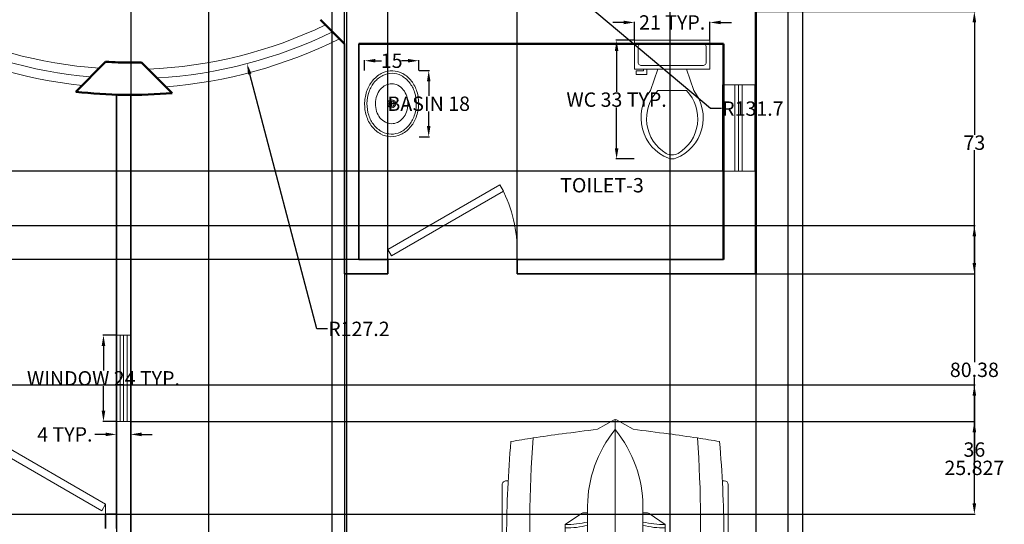
# Model space of a CAD drawing. Units: inches. Extents: x 1331 to 1798, y 701 to 1631.
# Tile 4 of 7: x 1524 to 1798, y 939 to 1079. Entities that reach past the tile are written whole.
import ezdxf

# ---------------------------------------------------------------- set-up
doc = ezdxf.new("R2010")
doc.units = ezdxf.units.IN
doc.header["$MEASUREMENT"] = 0
for name, color, linetype, lineweight in [('A-ANNO-DIMS', 2, 'Continuous', 18), ('A-AREA-IDEN', 7, 'Continuous', 18), ('A-EQPM-VEHI', 8, 'Continuous', 13), ('C-PROP', 7, 'Continuous', 25), ('DOORS', 241, 'Continuous', 18), ('INNER WALL', 50, 'Continuous', 35), ('OUTERWALL', 130, 'Continuous', 50), ('SANITARY', 1, 'Continuous', 18), ('VENTILATOR', 222, 'Continuous', 18), ('WINDOWS', 201, 'Continuous', 18)]:
    doc.layers.add(name, color=color, linetype=linetype, lineweight=lineweight)
doc.styles.get("Standard").update_dxf_attribs({"font": 'arial.ttf'})
doc.dimstyles.get("Standard").update_dxf_attribs({"dimtxt": 4, "dimasz": 3, "dimexe": 0.18, "dimexo": 0.0625, "dimgap": 0.09, "dimtad": 0, "dimtih": 1, "dimtoh": 1, "dimdec": 1, "dimzin": 0, "dimdsep": 46, "dimlunit": 3, "dimtxsty": 'Standard', "dimcen": 0.09, "dimadec": 0, "dimazin": 0, "dimtfac": 1, "dimtdec": 1, "dimtofl": 0, "dimtmove": 0, "dimatfit": 3, "dimfxl": 1, "dimtolj": 1, "dimtzin": 0, "dimarcsym": 0})

# ---------------------------------------------------------------- blocks, each defined once
blk = doc.blocks.new('*U12')
for p, q in [((0, 0), (0, -100)), ((750, 0), (750, -100))]:
    blk.add_line(p, q)
blk.add_lwpolyline([(0, 0), (649.5, 375), (671.4, 337.1), (21.9, -37.9)], close=True)
blk.add_arc((0, 0), 750, 0, 30)
blk = doc.blocks.new('*U14')
for p, q in [((0, 0), (0, 100)), ((750, 0), (750, 100))]:
    blk.add_line(p, q)
blk.add_lwpolyline([(0, 0), (649.5, -375), (671.4, -337.1), (21.9, 37.9)], close=True)
blk.add_arc((0, 0), 750, 330, 0)
blk = doc.blocks.new('Sink - Oval top')
for p, q in [((-1, 0), (1, 0)), ((0, 1), (0, -1))]:
    blk.add_line(p, q)
for points in [[(-12.23, 0.39, 0.117634), (-11.46, -3.36, 0.104469), (-8.88, -6.8, 0.090016), (-5.08, -9.07, 0.08192), (-0.32, -10.02, 0.08192), (4.49, -9.38, 0.090016), (8.42, -7.36, 0.104469), (11.22, -4.09, 0.117634), (12.23, -0.39, 0.117634), (11.46, 3.36, 0.104469), (8.88, 6.8, 0.090016), (5.08, 9.07, 0.08192), (0.32, 10.02, 0.08192), (-4.49, 9.38, 0.090016), (-8.42, 7.36, 0.104469), (-11.22, 4.09, 0.117634)], [(-11.29, 0.16, 0.118622), (-10.52, -3.25, 0.104678), (-8.07, -6.36, 0.089562), (-4.54, -8.37, 0.081185), (-0.13, -9.15, 0.081185), (4.3, -8.49, 0.089562), (7.89, -6.58, 0.104678), (10.42, -3.55, 0.118622), (11.29, -0.16, 0.118622), (10.52, 3.25, 0.104678), (8.07, 6.36, 0.089562), (4.54, 8.37, 0.081185), (0.13, 9.15, 0.081185), (-4.3, 8.49, 0.089562), (-7.89, 6.58, 0.104678), (-10.42, 3.55, 0.118622)], [(-7.42, 0.08, 0.118283), (-6.91, -2.17, 0.104607), (-5.29, -4.21, 0.089718), (-2.97, -5.53, 0.081436), (-0.07, -6.04, 0.081436), (2.84, -5.59, 0.089718), (5.2, -4.33, 0.104607), (6.86, -2.32, 0.118283), (7.42, -0.08, 0.118283), (6.91, 2.17, 0.104607), (5.29, 4.21, 0.089718), (2.97, 5.53, 0.081436), (0.07, 6.04, 0.081436), (-2.84, 5.59, 0.089718), (-5.2, 4.33, 0.104607), (-6.86, 2.32, 0.118283)]]:
    blk.add_lwpolyline(points, format="xyb", close=True)
for radius in [1.5, 1]:
    blk.add_circle((0, 0), radius)
blk = doc.blocks.new('*U17')
for p, q in [((21.1, 37.41), (21.1, 36.83)), ((46.55, 38.89), (22.35, 38.89)), ((47.8, 37.39), (47.8, 37.41)), ((135.45, 37.07), (135.45, 37.41)), ((136.7, 38.89), (160.9, 38.89)), ((162.15, 37.41), (162.15, 36.77)), ((87.99, 31.87), (74.76, 35.92)), ((134.31, 35.6), (119.29, 31.78)), ((70.03, 31.54), (86.41, 29.35)), ((186.47, -33.5), (186.47, 33.5)), ((188.4, -32.76), (188.4, 32.76)), ((138.42, 29.35), (157.25, 29.35)), ((186.47, 29.35), (167.01, 29.35)), ((164.52, 26.39), (164.52, -26.39)), ((32.27, 11.63), (36.13, 17.17)), ((36.13, 17.17), (50.94, 17.17)), ((32.12, 9.51), (32.12, 11.15)), ((58.92, -10.77), (58.92, 10.77)), ((66.55, -10.53), (66.55, 10.53)), ((186.47, -10.53), (186.47, 10.53)), ((29.77, 9.51), (51.68, 9.51)), ((82.74, 8.5), (82.74, -8.5)), ((3.27, 6.13), (0.1, 0.41)), ((0, 0), (51.68, 0)), ((0.1, -0.41), (3.27, -6.13)), ((29.77, -9.51), (51.68, -9.51)), ((32.12, -9.51), (32.12, -11.15)), ((32.27, -11.63), (36.13, -17.17)), ((36.13, -17.17), (50.94, -17.17)), ((86.41, -29.35), (70.03, -31.54)), ((157.25, -29.35), (138.42, -29.35)), ((167.01, -29.35), (186.47, -29.35)), ((87.99, -31.87), (74.76, -35.92)), ((134.31, -35.6), (119.29, -31.78)), ((21.1, -37.41), (21.1, -36.83)), ((135.45, -37.07), (135.45, -37.41)), ((162.15, -37.41), (162.15, -36.77)), ((46.55, -38.89), (22.35, -38.89)), ((47.8, -37.39), (47.8, -37.41)), ((136.7, -38.89), (160.9, -38.89))]:
    blk.add_line(p, q)
for centre, major_axis, ratio, start_param, end_param in [((41.19, -490.86), (0, 528.23), 0.842304, 0.00281, 0.075598), ((22.35, 37.41), (0, -1.48), 0.842304, 3.141593, 4.712389), ((64.48, -10555.62), (0, 10593.03), 0.842304, -0.013397, 0.002797), ((46.55, 37.41), (0, 1.48), 0.842304, -1.570796, 0), ((136.7, 37.41), (0, -1.48), 0.842304, 3.141593, 4.712389), ((160.9, 37.41), (0, 1.48), 0.842304, -1.570796, 0), ((180.63, 35.84), (0, 2.22), 0.842304, -0.013017, 1.249894), ((64.48, -10556.36), (0, 10595.31), 0.842304, -0.013397, -0.013017), ((183.98, 32.76), (0, -5.25), 0.842304, 1.570796, 3.128196), ((266.03, -27.52), (0, 313.31), 0.842304, 1.367076, 1.39176), ((64.48, -10555.62), (0, -10591.55), 0.842304, 3.133765, 3.140441), ((183.98, 33.5), (0, -2.96), 0.842304, 1.570796, 3.128196), ((135.29, 5.39), (0, 81.77), 0.842304, 1.245306, 1.50788), ((95.79, -3666.35), (0, -3698.24), 0.842304, 3.134049, 3.144098), ((259.18, -27.52), (0, -305.3), 0.842304, 4.528606, 4.561838), ((37.47, -593.96), (0, -623.33), 0.842304, 3.096046, 3.200911), ((134.4, 5.39), (0, -89.78), 0.842304, 4.449482, 4.652344), ((149.6, 2.8), (0, -79.58), 0.842304, 4.372215, 4.640744), ((17.08, 0), (0, 147.02), 0.842304, 4.511394, 4.913384), ((35.91, 0), (0, 147.02), 0.842304, 4.511394, 4.913384), ((167.01, 26.39), (0, 2.96), 0.842304, 0, 1.570796), ((-204.49, 52.4), (0, -250.96), 0.842304, 1.385369, 1.434372), ((13.04, 17.01), (0, 27.42), 0.842304, 4.435146, 4.718221), ((14.2, 17.01), (0, 27.42), 0.842304, 4.435146, 4.718221), ((50.79, 13.34), (6.34, -0.36), 0.603834, -1.395552, 1.581315), ((32.75, 11.15), (0, 0.74), 0.842304, 0.879714, 1.570796), ((29.77, -46.66), (0, 56.17), 0.842304, 0, 0.590319), ((0.62, 0), (0, -0.74), 0.842304, 4.131459, 5.293319), ((29.77, 46.66), (0, 56.17), 0.842304, 2.551274, 3.141593), ((-204.49, -52.4), (0, 250.96), 0.842304, -1.434372, -1.385369), ((13.04, -17.01), (0, -27.42), 0.842304, 1.564964, 1.848039), ((14.2, -17.01), (0, -27.42), 0.842304, 1.564964, 1.848039), ((149.6, -2.8), (0, -79.58), 0.842304, -1.499151, -1.230623), ((32.75, -11.15), (0, -0.74), 0.842304, 4.712389, 5.403472), ((134.4, -5.39), (0, -89.78), 0.842304, -1.510751, -1.307889), ((135.29, -5.39), (0, -81.77), 0.842304, -1.50788, -1.245306), ((259.18, 27.52), (0, 305.3), 0.842304, 1.721348, 1.754579), ((167.01, -26.39), (0, -2.96), 0.842304, 4.712389, 6.283185), ((266.03, 27.52), (0, 313.31), 0.842304, 1.749832, 1.774517), ((37.47, 593.96), (0, -623.33), 0.842304, -0.059319, 0.045547), ((95.79, 3666.35), (0, -3698.24), 0.842304, -0.002505, 0.007544), ((183.98, -33.5), (0, 2.96), 0.842304, 3.15499, 4.712389), ((183.98, -32.76), (0, -5.25), 0.842304, 0.013397, 1.570796), ((41.19, 490.86), (0, -528.23), 0.842304, -0.075598, -0.00281), ((64.48, 10555.62), (0, 10593.03), 0.842304, 3.138796, 3.15499), ((64.48, 10555.62), (0, -10591.55), 0.842304, 0.001152, 0.007828), ((180.63, -35.84), (0, -2.22), 0.842304, -1.249894, 0.013017), ((22.35, -37.41), (0, 1.48), 0.842304, 1.570796, 3.141593), ((46.55, -37.41), (0, -1.48), 0.842304, 0, 1.570796), ((136.7, -37.41), (0, -1.48), 0.842304, -1.570796, 0), ((160.9, -37.41), (0, 1.48), 0.842304, 3.141593, 4.712389), ((64.48, 10556.36), (0, 10595.31), 0.842304, 3.15461, 3.15499)]:
    blk.add_ellipse(centre, major_axis=major_axis, ratio=ratio, start_param=start_param, end_param=end_param)
at = {"extrusion": (0, 0, -1)}
blk.add_ellipse((50.79, -13.34), major_axis=(6.34, 0.36), ratio=0.603834, start_param=-1.395552, end_param=1.581315, dxfattribs=at)
blk = doc.blocks.new('Window - Wood Frame 36 in. Wide plan')
for p, q in [((0, 6), (0, 0)), ((0, 4.5), (36, 4.5)), ((36, 6), (36, 0)), ((0, 3), (36, 3)), ((0, 1.5), (36, 1.5))]:
    blk.add_line(p, q)
blk = doc.blocks.new('Toilet - top')
for p, q in [((9.5, -6), (9.5, -2)), ((-8, -8.5), (-8, -8)), ((-7, -8), (-7, -9.5)), ((-4, -8), (-6, -14)), ((4, -8), (6, -14)), ((-10, -8.5), (-8, -8.5)), ((-10, -9.5), (-10, -8.5)), ((-7, -9.5), (-10, -9.5)), ((4, -14), (-4, -14))]:
    blk.add_line(p, q)
blk.add_lwpolyline([(10.5, -8), (10.5, 0), (-10.5, 0), (-10.5, -8)], close=True)
for points in [[(-9.5, -2), (-9.5, -6)], [(8.5, -1), (-8.5, -1)], [(-8.5, -7), (8.5, -7)]]:
    blk.add_lwpolyline(points)
for centre, radius, start, end in [((-8.62, -1.88), 0.884, 81.8699, 188.1301), ((8.62, -1.88), 0.884, 351.8699, 98.1301), ((-8.62, -6.12), 0.884, 171.8699, 278.1301), ((8.62, -6.12), 0.884, 261.8699, 8.1301), ((3.52, -21.58), 12.17, 141.4691, 247.9714), ((4.2, -21.82), 11.33, 136.3677, 238.9468), ((-3.52, -21.58), 12.17, 292.0284, 38.5307), ((-4.2, -21.82), 11.33, 301.053, 43.6321), ((0, -27.88), 4, 245.7318, 294.2682), ((0, -29), 4, 254.8605, 285.1395)]:
    blk.add_arc(centre, radius, start, end)
blk = doc.blocks.new('VENT-FRAME-24IN')
for p, q in [((9, 24), (0, 24)), ((0, 24), (0, 0)), ((9, 0), (9, 24)), ((0, 0), (9, 0))]:
    blk.add_line(p, q)
blk = doc.blocks.new('*D26')
at = {"layer": 'A-ANNO-DIMS', "color": 0, "lineweight": -2, "transparency": 16777216}
for p, q in [((1550.6, 991.61), (1546.88, 991.61)), ((1547.06, 988.61), (1547.06, 981.77)), ((1547.06, 970.61), (1547.06, 977.46)), ((1550.6, 967.61), (1546.88, 967.61))]:
    blk.add_line(p, q, dxfattribs=at)
at = {"layer": 'A-ANNO-DIMS', "color": 0, "transparency": 16777216}
for points in [[(1546.56, 988.61), (1547.56, 988.61), (1547.06, 991.61)], [(1546.56, 970.61), (1547.56, 970.61), (1547.06, 967.61)]]:
    blk.add_solid(points, dxfattribs=at)
at = {"layer": 'Defpoints', "color": 0, "transparency": 16777216}
for p in [(1547.06, 991.61), (1550.66, 991.61), (1550.66, 967.61)]:
    blk.add_point(p, dxfattribs=at)
at = {"layer": 'A-ANNO-DIMS', "color": 0, "transparency": 16777216, "insert": (1547.06, 979.61), "char_height": 4, "attachment_point": 5}
blk.add_mtext('\\A1;WINDOW 24 TYP.', dxfattribs=at)
blk = doc.blocks.new('*D27')
at = {"layer": 'A-ANNO-DIMS', "color": 0, "lineweight": -2, "transparency": 16777216}
for p, q in [((1550.66, 967.55), (1550.66, 963.83)), ((1554.66, 967.55), (1554.66, 963.83)), ((1547.66, 964.01), (1544.66, 964.01)), ((1557.66, 964.01), (1560.66, 964.01))]:
    blk.add_line(p, q, dxfattribs=at)
at = {"layer": 'A-ANNO-DIMS', "color": 0, "transparency": 16777216}
for points in [[(1547.66, 964.51), (1547.66, 963.51), (1550.66, 964.01)], [(1557.66, 964.51), (1557.66, 963.51), (1554.66, 964.01)]]:
    blk.add_solid(points, dxfattribs=at)
at = {"layer": 'Defpoints', "color": 0, "transparency": 16777216}
for p in [(1550.66, 967.61), (1554.66, 967.61), (1550.66, 964.01)]:
    blk.add_point(p, dxfattribs=at)
at = {"layer": 'A-ANNO-DIMS', "color": 0, "transparency": 16777216, "insert": (1536.31, 964.01), "char_height": 4, "attachment_point": 5}
blk.add_mtext('\\A1;4 TYP.', dxfattribs=at)
blk = doc.blocks.new('*D36')
at = {"layer": 'A-ANNO-DIMS', "color": 0, "lineweight": -2, "transparency": 16777216}
for p, q in [((1634.88, 1065.25), (1637.76, 1065.25)), ((1637.58, 1062.25), (1637.58, 1058.2)), ((1637.58, 1049.83), (1637.58, 1053.88)), ((1634.88, 1046.83), (1637.76, 1046.83))]:
    blk.add_line(p, q, dxfattribs=at)
at = {"layer": 'A-ANNO-DIMS', "color": 0, "transparency": 16777216}
for points in [[(1637.08, 1062.25), (1638.08, 1062.25), (1637.58, 1065.25)], [(1637.08, 1049.83), (1638.08, 1049.83), (1637.58, 1046.83)]]:
    blk.add_solid(points, dxfattribs=at)
at = {"layer": 'Defpoints', "color": 0, "transparency": 16777216}
for p in [(1634.82, 1065.25), (1637.58, 1065.25), (1634.82, 1046.83)]:
    blk.add_point(p, dxfattribs=at)
at = {"layer": 'A-ANNO-DIMS', "color": 0, "transparency": 16777216, "insert": (1637.58, 1056.04), "char_height": 4, "attachment_point": 5}
blk.add_mtext('\\A1;BASIN 18', dxfattribs=at)
blk = doc.blocks.new('*D37')
at = {"layer": 'A-ANNO-DIMS', "color": 0, "lineweight": -2, "transparency": 16777216}
for p, q in [((1619.72, 1065.31), (1619.72, 1068.19)), ((1622.72, 1068.01), (1624.48, 1068.01)), ((1631.82, 1068.01), (1630.05, 1068.01)), ((1634.82, 1065.31), (1634.82, 1068.19))]:
    blk.add_line(p, q, dxfattribs=at)
at = {"layer": 'A-ANNO-DIMS', "color": 0, "transparency": 16777216}
for points in [[(1622.72, 1068.51), (1622.72, 1067.51), (1619.72, 1068.01)], [(1631.82, 1068.51), (1631.82, 1067.51), (1634.82, 1068.01)]]:
    blk.add_solid(points, dxfattribs=at)
at = {"layer": 'Defpoints', "color": 0, "transparency": 16777216}
for p in [(1619.72, 1068.01), (1619.72, 1065.25), (1634.82, 1065.25)]:
    blk.add_point(p, dxfattribs=at)
at = {"layer": 'A-ANNO-DIMS', "color": 0, "transparency": 16777216, "insert": (1627.27, 1068.01), "char_height": 4, "attachment_point": 5}
blk.add_mtext('\\A1;15', dxfattribs=at)
blk = doc.blocks.new('*D38')
at = {"layer": 'A-ANNO-DIMS', "color": 0, "lineweight": -2, "transparency": 16777216}
for p, q in [((1694.76, 1073.7), (1689.69, 1073.7)), ((1689.87, 1070.7), (1689.87, 1059.34)), ((1689.87, 1043.66), (1689.87, 1055.02)), ((1694.76, 1040.66), (1689.69, 1040.66))]:
    blk.add_line(p, q, dxfattribs=at)
at = {"layer": 'A-ANNO-DIMS', "color": 0, "transparency": 16777216}
for points in [[(1689.37, 1070.7), (1690.37, 1070.7), (1689.87, 1073.7)], [(1689.37, 1043.66), (1690.37, 1043.66), (1689.87, 1040.66)]]:
    blk.add_solid(points, dxfattribs=at)
at = {"layer": 'Defpoints', "color": 0, "transparency": 16777216}
for p in [(1689.87, 1073.7), (1694.83, 1073.7), (1694.83, 1040.66)]:
    blk.add_point(p, dxfattribs=at)
at = {"layer": 'A-ANNO-DIMS', "color": 0, "transparency": 16777216, "insert": (1689.87, 1057.18), "char_height": 4, "attachment_point": 5}
blk.add_mtext('\\A1;WC 33 TYP.', dxfattribs=at)
blk = doc.blocks.new('*D39')
at = {"layer": 'A-ANNO-DIMS', "color": 0, "lineweight": -2, "transparency": 16777216}
for p, q in [((1691.83, 1078.66), (1688.83, 1078.66)), ((1694.83, 1073.77), (1694.83, 1078.84)), ((1715.83, 1073.77), (1715.83, 1078.84)), ((1718.83, 1078.66), (1721.83, 1078.66))]:
    blk.add_line(p, q, dxfattribs=at)
at = {"layer": 'A-ANNO-DIMS', "color": 0, "transparency": 16777216}
for points in [[(1691.83, 1079.16), (1691.83, 1078.16), (1694.83, 1078.66)], [(1718.83, 1079.16), (1718.83, 1078.16), (1715.83, 1078.66)]]:
    blk.add_solid(points, dxfattribs=at)
at = {"layer": 'Defpoints', "color": 0, "transparency": 16777216}
for p in [(1715.83, 1078.66), (1694.83, 1073.7), (1715.83, 1073.7)]:
    blk.add_point(p, dxfattribs=at)
at = {"layer": 'A-ANNO-DIMS', "color": 0, "transparency": 16777216, "insert": (1705.33, 1078.66), "char_height": 4, "attachment_point": 5}
blk.add_mtext('\\A1;21 TYP.', dxfattribs=at)
blk = doc.blocks.new('*D55')
at = {"layer": 'A-ANNO-DIMS', "color": 0, "lineweight": -2, "transparency": 16777216}
for p, q in [((1554.66, 1190.15), (1554.66, 703.35)), ((1728.66, 1008.64), (1728.66, 703.35)), ((1557.66, 703.53), (1637.35, 703.53)), ((1725.66, 703.53), (1645.98, 703.53))]:
    blk.add_line(p, q, dxfattribs=at)
at = {"layer": 'A-ANNO-DIMS', "color": 0, "transparency": 16777216}
for points in [[(1557.66, 704.03), (1557.66, 703.03), (1554.66, 703.53)], [(1725.66, 704.03), (1725.66, 703.03), (1728.66, 703.53)]]:
    blk.add_solid(points, dxfattribs=at)
at = {"layer": 'Defpoints', "color": 0, "transparency": 16777216}
for p in [(1554.66, 1190.21), (1728.66, 1008.7), (1728.66, 703.53)]:
    blk.add_point(p, dxfattribs=at)
at = {"layer": 'A-ANNO-DIMS', "color": 0, "transparency": 16777216, "insert": (1641.66, 703.53), "char_height": 4, "attachment_point": 5}
blk.add_mtext('\\A1;174', dxfattribs=at)
blk = doc.blocks.new('*D61')
at = {"layer": 'A-ANNO-DIMS', "color": 0, "lineweight": -2, "transparency": 16777216}
for p, q in [((1554.663699, 1524.863082), (1554.663699, 703.345582)), ((1576.268161, 1524.863082), (1576.268161, 703.345582)), ((1551.663699, 703.525582), (1548.663699, 703.525582)), ((1579.268161, 703.525582), (1582.268161, 703.525582))]:
    blk.add_line(p, q, dxfattribs=at)
at = {"layer": 'A-ANNO-DIMS', "color": 0, "transparency": 16777216}
for points in [[(1551.663699, 704.025582), (1551.663699, 703.025582), (1554.663699, 703.525582)], [(1579.268161, 704.025582), (1579.268161, 703.025582), (1576.268161, 703.525582)]]:
    blk.add_solid(points, dxfattribs=at)
at = {"layer": 'Defpoints', "color": 0, "transparency": 16777216}
for p in [(1554.663699, 1524.925582), (1576.268161, 1524.925582), (1576.268161, 703.525582)]:
    blk.add_point(p, dxfattribs=at)
at = {"layer": 'A-ANNO-DIMS', "color": 0, "transparency": 16777216, "insert": (1565.46593, 703.525582), "char_height": 4, "attachment_point": 5}
blk.add_mtext('\\A1;21.604', dxfattribs=at)
blk = doc.blocks.new('*D69')
at = {"layer": 'A-ANNO-DIMS', "color": 0, "lineweight": -2, "transparency": 16777216}
for p, q in [((1614.66, 1376.86), (1614.66, 703.35)), ((1704.66, 1376.86), (1704.66, 703.35)), ((1617.66, 703.53), (1656.72, 703.53)), ((1701.66, 703.53), (1662.61, 703.53))]:
    blk.add_line(p, q, dxfattribs=at)
at = {"layer": 'A-ANNO-DIMS', "color": 0, "transparency": 16777216}
for points in [[(1617.66, 704.03), (1617.66, 703.03), (1614.66, 703.53)], [(1701.66, 704.03), (1701.66, 703.03), (1704.66, 703.53)]]:
    blk.add_solid(points, dxfattribs=at)
at = {"layer": 'Defpoints', "color": 0, "transparency": 16777216}
for p in [(1614.66, 1376.93), (1704.66, 1376.93), (1704.66, 703.53)]:
    blk.add_point(p, dxfattribs=at)
at = {"layer": 'A-ANNO-DIMS', "color": 0, "transparency": 16777216, "insert": (1659.66, 703.53), "char_height": 4, "attachment_point": 5}
blk.add_mtext('\\A1;90', dxfattribs=at)
blk = doc.blocks.new('*D71')
at = {"layer": 'A-ANNO-DIMS', "color": 0, "lineweight": -2, "transparency": 16777216}
for p, q in [((1506.66, 1376.86), (1506.66, 703.35)), ((1610.66, 1376.86), (1610.66, 703.35)), ((1509.66, 703.53), (1554.35, 703.53)), ((1607.66, 703.53), (1562.98, 703.53))]:
    blk.add_line(p, q, dxfattribs=at)
at = {"layer": 'A-ANNO-DIMS', "color": 0, "transparency": 16777216}
for points in [[(1509.66, 704.03), (1509.66, 703.03), (1506.66, 703.53)], [(1607.66, 704.03), (1607.66, 703.03), (1610.66, 703.53)]]:
    blk.add_solid(points, dxfattribs=at)
at = {"layer": 'Defpoints', "color": 0, "transparency": 16777216}
for p in [(1506.66, 1376.93), (1610.66, 1376.93), (1610.66, 703.53)]:
    blk.add_point(p, dxfattribs=at)
at = {"layer": 'A-ANNO-DIMS', "color": 0, "transparency": 16777216, "insert": (1558.66, 703.53), "char_height": 4, "attachment_point": 5}
blk.add_mtext('\\A1;104', dxfattribs=at)
blk = doc.blocks.new('*D75')
at = {"layer": 'A-ANNO-DIMS', "color": 0, "lineweight": -2, "transparency": 16777216}
for p, q in [((1418.66, 941.73), (1418.66, 703.35)), ((1550.66, 941.73), (1550.66, 703.35)), ((1421.66, 703.53), (1480.36, 703.53)), ((1547.66, 703.53), (1488.96, 703.53))]:
    blk.add_line(p, q, dxfattribs=at)
at = {"layer": 'A-ANNO-DIMS', "color": 0, "transparency": 16777216}
for points in [[(1421.66, 704.03), (1421.66, 703.03), (1418.66, 703.53)], [(1547.66, 704.03), (1547.66, 703.03), (1550.66, 703.53)]]:
    blk.add_solid(points, dxfattribs=at)
at = {"layer": 'Defpoints', "color": 0, "transparency": 16777216}
for p in [(1418.66, 941.79), (1550.66, 941.79), (1550.66, 703.53)]:
    blk.add_point(p, dxfattribs=at)
at = {"layer": 'A-ANNO-DIMS', "color": 0, "transparency": 16777216, "insert": (1484.66, 703.53), "char_height": 4, "attachment_point": 5}
blk.add_mtext('\\A1;132', dxfattribs=at)
blk = doc.blocks.new('*D79')
at = {"layer": 'A-ANNO-DIMS', "color": 0, "lineweight": -2, "transparency": 16777216}
for p, q in [((1554.73, 967.61), (1789.62, 967.61)), ((1789.44, 964.61), (1789.44, 956.83)), ((1789.44, 944.79), (1789.44, 952.57)), ((1550.73, 941.79), (1789.62, 941.79))]:
    blk.add_line(p, q, dxfattribs=at)
at = {"layer": 'A-ANNO-DIMS', "color": 0, "transparency": 16777216}
for points in [[(1788.94, 964.61), (1789.94, 964.61), (1789.44, 967.61)], [(1788.94, 944.79), (1789.94, 944.79), (1789.44, 941.79)]]:
    blk.add_solid(points, dxfattribs=at)
at = {"layer": 'Defpoints', "color": 0, "transparency": 16777216}
for p in [(1554.66, 967.61), (1789.44, 967.61), (1550.66, 941.79)]:
    blk.add_point(p, dxfattribs=at)
at = {"layer": 'A-ANNO-DIMS', "color": 0, "transparency": 16777216, "insert": (1789.44, 954.7), "char_height": 4, "attachment_point": 5}
blk.add_mtext('\\A1;25.827', dxfattribs=at)
blk = doc.blocks.new('*D82')
at = {"layer": 'A-ANNO-DIMS', "color": 0, "lineweight": -2, "transparency": 16777216}
for p, q in [((1418.73, 1022.17), (1789.62, 1022.17)), ((1789.44, 1019.17), (1789.44, 984.11)), ((1789.44, 944.79), (1789.44, 979.84)), ((1418.73, 941.79), (1789.62, 941.79))]:
    blk.add_line(p, q, dxfattribs=at)
at = {"layer": 'A-ANNO-DIMS', "color": 0, "transparency": 16777216}
for points in [[(1788.94, 1019.17), (1789.94, 1019.17), (1789.44, 1022.17)], [(1788.94, 944.79), (1789.94, 944.79), (1789.44, 941.79)]]:
    blk.add_solid(points, dxfattribs=at)
at = {"layer": 'Defpoints', "color": 0, "transparency": 16777216}
for p in [(1418.66, 1022.17), (1789.44, 1022.17), (1418.66, 941.79)]:
    blk.add_point(p, dxfattribs=at)
at = {"layer": 'A-ANNO-DIMS', "color": 0, "transparency": 16777216, "insert": (1789.44, 981.98), "char_height": 4, "attachment_point": 5}
blk.add_mtext('\\A1;80.38', dxfattribs=at)
blk = doc.blocks.new('*D84')
at = {"layer": 'A-ANNO-DIMS', "color": 0, "lineweight": -2, "transparency": 16777216}
for p, q in [((1493.13, 977.79), (1789.62, 977.79)), ((1789.44, 974.79), (1789.44, 961.92)), ((1789.44, 944.79), (1789.44, 957.65)), ((1493.13, 941.79), (1789.62, 941.79))]:
    blk.add_line(p, q, dxfattribs=at)
at = {"layer": 'A-ANNO-DIMS', "color": 0, "transparency": 16777216}
for points in [[(1788.94, 974.79), (1789.94, 974.79), (1789.44, 977.79)], [(1788.94, 944.79), (1789.94, 944.79), (1789.44, 941.79)]]:
    blk.add_solid(points, dxfattribs=at)
at = {"layer": 'Defpoints', "color": 0, "transparency": 16777216}
for p in [(1493.07, 977.79), (1789.44, 977.79), (1493.07, 941.79)]:
    blk.add_point(p, dxfattribs=at)
at = {"layer": 'A-ANNO-DIMS', "color": 0, "transparency": 16777216, "insert": (1789.44, 959.79), "char_height": 4, "attachment_point": 5}
blk.add_mtext('\\A1;36', dxfattribs=at)
blk = doc.blocks.new('*D85')
at = {"layer": 'A-ANNO-DIMS', "color": 0, "lineweight": -2, "transparency": 16777216}
for p, q in [((1614.16, 1008.64), (1614.16, 703.35)), ((1728.66, 1008.64), (1728.66, 703.35)), ((1617.16, 703.53), (1664.75, 703.53)), ((1725.66, 703.53), (1678.08, 703.53))]:
    blk.add_line(p, q, dxfattribs=at)
at = {"layer": 'A-ANNO-DIMS', "color": 0, "transparency": 16777216}
for points in [[(1617.16, 704.03), (1617.16, 703.03), (1614.16, 703.53)], [(1725.66, 704.03), (1725.66, 703.03), (1728.66, 703.53)]]:
    blk.add_solid(points, dxfattribs=at)
at = {"layer": 'Defpoints', "color": 0, "transparency": 16777216}
for p in [(1614.16, 1008.7), (1728.66, 1008.7), (1728.66, 703.53)]:
    blk.add_point(p, dxfattribs=at)
at = {"layer": 'A-ANNO-DIMS', "color": 0, "transparency": 16777216, "insert": (1671.41, 703.53), "char_height": 4, "attachment_point": 5}
blk.add_mtext('\\A1;114.5', dxfattribs=at)
blk = doc.blocks.new('*D86')
at = {"layer": 'A-ANNO-DIMS', "color": 0, "lineweight": -2, "transparency": 16777216}
for p, q in [((1728.73, 1081.7), (1789.62, 1081.7)), ((1789.44, 1078.7), (1789.44, 1047.34)), ((1789.44, 1011.7), (1789.44, 1043.07)), ((1728.73, 1008.7), (1789.62, 1008.7))]:
    blk.add_line(p, q, dxfattribs=at)
at = {"layer": 'A-ANNO-DIMS', "color": 0, "transparency": 16777216}
for points in [[(1788.94, 1078.7), (1789.94, 1078.7), (1789.44, 1081.7)], [(1788.94, 1011.7), (1789.94, 1011.7), (1789.44, 1008.7)]]:
    blk.add_solid(points, dxfattribs=at)
at = {"layer": 'Defpoints', "color": 0, "transparency": 16777216}
for p in [(1728.66, 1081.7), (1789.44, 1081.7), (1728.66, 1008.7)]:
    blk.add_point(p, dxfattribs=at)
at = {"layer": 'A-ANNO-DIMS', "color": 0, "transparency": 16777216, "insert": (1789.44, 1045.2), "char_height": 4, "attachment_point": 5}
blk.add_mtext('\\A1;73', dxfattribs=at)
blk = doc.blocks.new('*D87')
at = {"layer": 'A-ANNO-DIMS', "color": 0, "lineweight": -2, "transparency": 16777216}
for p, q in [((1626.16, 1008.77), (1626.16, 1628.51)), ((1629.16, 1628.33), (1641.21, 1628.33)), ((1659.16, 1628.33), (1647.12, 1628.33)), ((1662.16, 1008.77), (1662.16, 1628.51))]:
    blk.add_line(p, q, dxfattribs=at)
at = {"layer": 'A-ANNO-DIMS', "color": 0, "transparency": 16777216}
for points in [[(1629.16, 1628.83), (1629.16, 1627.83), (1626.16, 1628.33)], [(1659.16, 1628.83), (1659.16, 1627.83), (1662.16, 1628.33)]]:
    blk.add_solid(points, dxfattribs=at)
at = {"layer": 'Defpoints', "color": 0, "transparency": 16777216}
for p in [(1662.16, 1628.33), (1626.16, 1008.7), (1662.16, 1008.7)]:
    blk.add_point(p, dxfattribs=at)
at = {"layer": 'A-ANNO-DIMS', "color": 0, "transparency": 16777216, "insert": (1644.16, 1628.33), "char_height": 4, "attachment_point": 5}
blk.add_mtext('\\A1;36', dxfattribs=at)
blk = doc.blocks.new('*D88')
at = {"layer": 'A-ANNO-DIMS', "color": 0, "lineweight": -2, "transparency": 16777216}
for p, q in [((1614.16, 1008.77), (1614.16, 1628.51)), ((1617.16, 1628.33), (1617.42, 1628.33)), ((1623.16, 1628.33), (1622.91, 1628.33)), ((1626.16, 1008.77), (1626.16, 1628.51))]:
    blk.add_line(p, q, dxfattribs=at)
at = {"layer": 'A-ANNO-DIMS', "color": 0, "transparency": 16777216}
for points in [[(1617.16, 1628.83), (1617.16, 1627.83), (1614.16, 1628.33)], [(1623.16, 1628.83), (1623.16, 1627.83), (1626.16, 1628.33)]]:
    blk.add_solid(points, dxfattribs=at)
at = {"layer": 'Defpoints', "color": 0, "transparency": 16777216}
for p in [(1626.16, 1628.33), (1614.16, 1008.7), (1626.16, 1008.7)]:
    blk.add_point(p, dxfattribs=at)
at = {"layer": 'A-ANNO-DIMS', "color": 0, "transparency": 16777216, "insert": (1620.16, 1628.33), "char_height": 4, "attachment_point": 5}
blk.add_mtext('\\A1;12', dxfattribs=at)
blk = doc.blocks.new('*D89')
at = {"layer": 'A-ANNO-DIMS', "color": 0, "lineweight": -2, "transparency": 16777216}
for p, q in [((1719.26, 1037.31), (1339.08, 1037.31)), ((1339.26, 1034.31), (1339.26, 1027.14)), ((1339.26, 1015.7), (1339.26, 1022.88)), ((1719.6, 1012.7), (1339.08, 1012.7))]:
    blk.add_line(p, q, dxfattribs=at)
at = {"layer": 'A-ANNO-DIMS', "color": 0, "transparency": 16777216}
for points in [[(1338.76, 1034.31), (1339.76, 1034.31), (1339.26, 1037.31)], [(1338.76, 1015.7), (1339.76, 1015.7), (1339.26, 1012.7)]]:
    blk.add_solid(points, dxfattribs=at)
at = {"layer": 'Defpoints', "color": 0, "transparency": 16777216}
for p in [(1339.26, 1037.31), (1719.32, 1037.31), (1719.66, 1012.7)]:
    blk.add_point(p, dxfattribs=at)
at = {"layer": 'A-ANNO-DIMS', "color": 0, "transparency": 16777216, "insert": (1339.26, 1025.01), "char_height": 4, "attachment_point": 5}
blk.add_mtext('\\A1;24.61', dxfattribs=at)
blk = doc.blocks.new('*D90')
at = {"layer": 'A-ANNO-DIMS', "color": 0, "lineweight": -2, "transparency": 16777216}
for p, q in [((1554.66, 1190.15), (1554.66, 703.35)), ((1409.66, 805.73), (1409.66, 703.35)), ((1412.66, 703.53), (1477.83, 703.53)), ((1551.66, 703.53), (1486.5, 703.53))]:
    blk.add_line(p, q, dxfattribs=at)
at = {"layer": 'A-ANNO-DIMS', "color": 0, "transparency": 16777216}
for points in [[(1412.66, 704.03), (1412.66, 703.03), (1409.66, 703.53)], [(1551.66, 704.03), (1551.66, 703.03), (1554.66, 703.53)]]:
    blk.add_solid(points, dxfattribs=at)
at = {"layer": 'Defpoints', "color": 0, "transparency": 16777216}
for p in [(1554.66, 1190.21), (1409.66, 805.79), (1554.66, 703.53)]:
    blk.add_point(p, dxfattribs=at)
at = {"layer": 'A-ANNO-DIMS', "color": 0, "transparency": 16777216, "insert": (1482.16, 703.53), "char_height": 4, "attachment_point": 5}
blk.add_mtext('\\A1;145', dxfattribs=at)
blk = doc.blocks.new('*D98')
at = {"layer": 'A-ANNO-DIMS', "color": 0, "lineweight": -2, "transparency": 16777216}
for p, q in [((1554.57, 1190.21), (1554.75, 1190.21)), ((1554.66, 1190.12), (1554.66, 1190.3)), ((1716.04, 1054.68), (1657.82, 1103.57)), ((1719.04, 1054.68), (1716.04, 1054.68))]:
    blk.add_line(p, q, dxfattribs=at)
at = {"layer": 'A-ANNO-DIMS', "color": 0, "transparency": 16777216}
blk.add_solid([(1658.14, 1103.96), (1657.5, 1103.19), (1655.52, 1105.5)], dxfattribs=at)
at = {"layer": 'Defpoints', "color": 0, "transparency": 16777216}
for p in [(1554.66, 1190.21), (1655.52, 1105.5)]:
    blk.add_point(p, dxfattribs=at)
at = {"layer": 'A-ANNO-DIMS', "color": 0, "transparency": 16777216, "insert": (1727.79, 1054.68), "char_height": 4, "attachment_point": 5}
blk.add_mtext('\\A1;R131.7', dxfattribs=at)
blk = doc.blocks.new('*D106')
at = {"layer": 'A-ANNO-DIMS', "color": 0, "lineweight": -2, "transparency": 16777216}
for p, q in [((1554.57, 1190.21), (1554.75, 1190.21)), ((1554.66, 1190.12), (1554.66, 1190.3)), ((1606.43, 993.38), (1587.78, 1064.29)), ((1609.43, 993.38), (1606.43, 993.38))]:
    blk.add_line(p, q, dxfattribs=at)
at = {"layer": 'A-ANNO-DIMS', "color": 0, "transparency": 16777216}
blk.add_solid([(1588.26, 1064.42), (1587.3, 1064.16), (1587.02, 1067.19)], dxfattribs=at)
at = {"layer": 'Defpoints', "color": 0, "transparency": 16777216}
for p in [(1554.66, 1190.21), (1587.02, 1067.19)]:
    blk.add_point(p, dxfattribs=at)
at = {"layer": 'A-ANNO-DIMS', "color": 0, "transparency": 16777216, "insert": (1618.16, 993.38), "char_height": 4, "attachment_point": 5}
blk.add_mtext('\\A1;R127.2', dxfattribs=at)

msp = doc.modelspace()

# ---------------------------------------------------------------- linework, layer by layer
at = {"layer": 'C-PROP'}
for p, q in [((1737.6637, 745.9256), (1737.6637, 1081.7042)), ((1737.6637, 749.9256), (1737.6637, 967.7042))]:
    msp.add_line(p, q, dxfattribs=at)
msp.add_lwpolyline([(1737.6637, 745.9256), (1741.6637, 745.9256), (1741.6637, 1585.9256), (1381.6637, 1585.9256), (1381.6637, 745.9256), (1559.6637, 745.9256)], dxfattribs=at)
msp.add_lwpolyline([(1737.6637, 745.9256), (1741.6637, 745.9256), (1741.6637, 1585.9256), (1381.6637, 1585.9256), (1381.6637, 745.9256), (1559.6637, 745.9256)], dxfattribs=at)
at = {"layer": 'DOORS'}
for radius, start, end in [(127.2045, 242.746718, 264.952813), (124.6123, 243.128584, 265.958714), (124.6123, 272.210712, 295.780765), (129.8022, 242.380125, 263.998895), (127.2045, 273.282313, 296.187311), (129.8022, 274.296605, 296.577489)]:
    msp.add_arc((1554.6637, 1190.2129), radius, start, end, dxfattribs=at)
at = {"layer": 'INNER WALL'}
for p, q in [((1614.1637, 1008.7042), (1614.1637, 1072.7042)), ((1618.1637, 1012.7042), (1618.1637, 1072.7042)), ((1550.6637, 1058.561), (1550.6637, 941.7881)), ((1554.6637, 1058.5002), (1554.6637, 805.7881)), ((1618.1637, 1012.7042), (1626.1637, 1012.7042)), ((1626.1637, 1008.7042), (1626.1637, 1012.7042)), ((1662.1637, 1008.7042), (1662.1637, 1012.7042)), ((1662.1637, 1012.7042), (1719.6637, 1012.7042)), ((1614.1637, 1008.7042), (1626.1637, 1008.7042)), ((1662.1637, 1008.7042), (1728.6637, 1008.7042)), ((1550.6637, 941.7881), (1547.6637, 941.7881)), ((1547.6637, 941.7881), (1547.6637, 937.7881)), ((1550.6637, 941.7881), (1550.6637, 937.7881))]:
    msp.add_line(p, q, dxfattribs=at)
at = {"layer": 'OUTERWALL'}
for p, q in [((1728.6637, 1008.7042), (1728.6637, 1081.7042)), ((1614.1609, 1072.7042), (1607.4373, 1079.4278)), ((1614.1609, 1072.7042), (1614.1637, 1072.7042)), ((1618.1637, 1072.7042), (1719.6637, 1072.7042)), ((1719.6637, 1012.7042), (1719.6637, 1072.7042)), ((1547.6708, 1067.6997), (1539.3631, 1059.392)), ((1554.6637, 1067.5002), (1557.6637, 1067.5002)), ((1557.6637, 1067.5002), (1566.1609, 1059.003))]:
    msp.add_line(p, q, dxfattribs=at)
for radius, start, end in [(122.7127, 266.733174, 270), (131.7127, 263.329094, 275.00774)]:
    msp.add_arc((1554.6637, 1190.2129), radius, start, end, dxfattribs=at)

# ---------------------------------------------------------------- block references
at = {"layer": 'A-EQPM-VEHI', "xscale": 0.8092702338706128, "yscale": 0.8092702338706128, "zscale": 0.8092702338706128, "rotation": 270}
msp.add_blockref('*U17', (1689.4906, 968.1545), dxfattribs=at)
at = {"layer": 'DOORS', "xscale": 0.0479999999999999, "yscale": 0.0479999999999999, "zscale": 0.0479999999999999}
msp.add_blockref('*U12', (1626.1637, 1015.5042), dxfattribs=at)
at = {"layer": 'DOORS', "xscale": 0.0479999999999998, "yscale": 0.0479999999999998, "zscale": 0.0479999999999998, "rotation": 180}
msp.add_blockref('*U14', (1547.6637, 944.5881), dxfattribs=at)
at = {"layer": 'SANITARY'}
msp.add_blockref('Toilet - top', (1705.3264, 1073.7042), dxfattribs=at)
at = {"layer": 'SANITARY', "xscale": 0.75, "yscale": 0.75, "zscale": 0.75, "rotation": 90}
msp.add_blockref('Sink - Oval top', (1627.2666, 1056.0395), dxfattribs=at)
at = {"layer": 'VENTILATOR'}
msp.add_blockref('VENT-FRAME-24IN', (1719.3197, 1037.3125), dxfattribs=at)
at = {"layer": 'VENTILATOR', "xscale": 0.6666666666666683, "yscale": 0.6666666666666683, "zscale": 0.6666666666666683, "rotation": 90}
msp.add_blockref('Window - Wood Frame 36 in. Wide plan', (1725.8194, 1037.3127), dxfattribs=at)
at = {"layer": 'WINDOWS', "xscale": 0.666666666666667, "yscale": 0.666666666666667, "zscale": 0.666666666666667, "rotation": 90}
msp.add_blockref('Window - Wood Frame 36 in. Wide plan', (1554.6637, 967.6148), dxfattribs=at)

# ---------------------------------------------------------------- texts
at = {"layer": 'A-AREA-IDEN', "insert": (1674.1605, 1035.3542), "char_height": 4, "attachment_point": 1}
msp.add_mtext_dynamic_manual_height_columns('TOILET-3', width=10.426026, gutter_width=1, heights=[1.7577], dxfattribs=at)

# ---------------------------------------------------------------- dimensions: what is measured, and where the dimension line sits
at = {"layer": 'A-ANNO-DIMS'}
for base, p1, p2, override, picture, middle in [((1626.1637, 1628.3256), (1614.1637, 1008.7042), (1626.1637, 1008.7042), {"dimdec": 0, "dimlfac": 1, "dimrnd": 0, "dimzin": 0, "dimdsep": 46, "dimlunit": 2}, '*D88', (1620.1637, 1628.3256)), ((1662.1637, 1628.3256), (1626.1637, 1008.7042), (1662.1637, 1008.7042), {"dimdec": 0, "dimlfac": 1, "dimrnd": 0, "dimzin": 0, "dimdsep": 46, "dimlunit": 2}, '*D87', (1644.1637, 1628.3256)), ((1576.26816, 703.52558), (1554.6637, 1524.92558), (1576.26816, 1524.92558), {"dimdec": 3, "dimlfac": 1, "dimrnd": 0, "dimzin": 0, "dimdsep": 46, "dimlunit": 2}, '*D61', (1565.46593, 703.52558)), ((1610.6637, 703.5256), (1506.6637, 1376.9256), (1610.6637, 1376.9256), {"dimdec": 0, "dimlfac": 1, "dimrnd": 0, "dimzin": 0, "dimdsep": 46, "dimlunit": 2}, '*D71', (1558.6637, 703.5256)), ((1704.6637, 703.5256), (1614.6637, 1376.9256), (1704.6637, 1376.9256), {"dimdec": 0, "dimlfac": 1, "dimrnd": 0, "dimzin": 0, "dimdsep": 46, "dimlunit": 2}, '*D69', (1659.6637, 703.5256)), ((1554.6637, 703.5256), (1409.6637, 805.7881), (1554.6637, 1190.2129), {"dimdec": 0, "dimlfac": 1, "dimrnd": 0, "dimzin": 0, "dimdsep": 46, "dimlunit": 2}, '*D90', (1482.1637, 703.5256)), ((1728.6637, 703.5256), (1554.6637, 1190.2129), (1728.6637, 1008.7042), {"dimdec": 0, "dimlfac": 1, "dimrnd": 0, "dimzin": 0, "dimdsep": 46, "dimlunit": 2}, '*D55', (1641.6637, 703.5256)), ((1728.6637, 703.5256), (1614.1637, 1008.7042), (1728.6637, 1008.7042), {"dimdec": 1, "dimlfac": 1, "dimrnd": 0, "dimzin": 0, "dimdsep": 46, "dimlunit": 2}, '*D85', (1671.4137, 703.5256)), ((1550.6637, 703.5256), (1418.6637, 941.7881), (1550.6637, 941.7881), {"dimdec": 0, "dimlfac": 1, "dimrnd": 0, "dimzin": 0, "dimdsep": 46, "dimlunit": 2}, '*D75', (1484.6637, 703.5256))]:
    dim = msp.add_linear_dim(base=base, p1=p1, p2=p2, dimstyle='Standard', override=override, dxfattribs=at)
    dim.commit()
    dim.dimension.update_dxf_attribs({"geometry": picture, "text_midpoint": middle})
for mpoint, picture, middle in [((1655.5216, 1105.5022), '*D98', (1727.7894, 1054.6758)), ((1587.0181, 1067.1918), '*D106', (1618.1632, 993.3791))]:
    dim = msp.add_radius_dim(center=(1554.6637, 1190.2129), mpoint=mpoint, dimstyle='Standard', override={"dimdec": 1, "dimlfac": 1, "dimrnd": 0, "dimzin": 0, "dimdsep": 46, "dimlunit": 2}, dxfattribs=at)
    dim.commit()
    dim.dimension.update_dxf_attribs({"geometry": picture, "text_midpoint": middle, "dimtype": 164})
dim = msp.add_linear_dim(base=(1715.8264, 1078.6611), p1=(1694.8264, 1073.7042), p2=(1715.8264, 1073.7042), text='<> TYP.', dimstyle='Standard', override={"dimdec": 0, "dimlfac": 1, "dimrnd": 0, "dimzin": 0, "dimdsep": 46, "dimlunit": 2}, dxfattribs=at)
dim.commit()
dim.dimension.update_dxf_attribs({"geometry": '*D39', "text_midpoint": (1705.3264, 1078.6611)})
for base, p1, p2, angle, override, picture, middle in [((1789.4411, 1081.7042), (1728.6637, 1008.7042), (1728.6637, 1081.7042), 90, {"dimdec": 0, "dimlfac": 1, "dimrnd": 0, "dimzin": 0, "dimdsep": 46, "dimlunit": 2}, '*D86', (1789.4411, 1045.2042)), ((1619.7154, 1068.0081), (1634.8178, 1065.2461), (1619.7154, 1065.2461), 180, {"dimdec": 0, "dimlfac": 1, "dimrnd": 0, "dimzin": 0, "dimdsep": 46, "dimlunit": 2}, '*D37', (1627.2666, 1068.0081)), ((1339.2637, 1037.3127), (1719.6637, 1012.7042), (1719.3194, 1037.3127), 90, {"dimdec": 2, "dimlfac": 1, "dimrnd": 0, "dimzin": 0, "dimdsep": 46, "dimlunit": 2}, '*D89', (1339.2637, 1025.0084)), ((1789.4411, 1022.1692), (1418.6637, 941.7881), (1418.6637, 1022.1692), 90, {"dimdec": 2, "dimlfac": 1, "dimrnd": 0, "dimzin": 0, "dimdsep": 46, "dimlunit": 2}, '*D82', (1789.4411, 981.9786)), ((1789.4411, 977.7881), (1493.0724, 941.7881), (1493.0724, 977.7881), 90, {"dimdec": 0, "dimlfac": 1, "dimrnd": 0, "dimzin": 0, "dimdsep": 46, "dimlunit": 2}, '*D84', (1789.4411, 959.7881)), ((1789.4411, 967.6148), (1550.6637, 941.7881), (1554.6637, 967.6148), 90, {"dimdec": 3, "dimlfac": 1, "dimrnd": 0, "dimzin": 0, "dimdsep": 46, "dimlunit": 2}, '*D79', (1789.4411, 954.7014))]:
    dim = msp.add_linear_dim(base=base, p1=p1, p2=p2, angle=angle, dimstyle='Standard', override=override, dxfattribs=at)
    dim.commit()
    dim.dimension.update_dxf_attribs({"geometry": picture, "text_midpoint": middle})
for base, p1, p2, angle, text, picture, middle in [((1689.8694, 1073.7042), (1694.8264, 1040.6579), (1694.8264, 1073.7042), 90, 'WC <> TYP.', '*D38', (1689.8694, 1057.181)), ((1637.5798, 1065.2461), (1634.8178, 1046.833), (1634.8178, 1065.2461), 90, 'BASIN <>', '*D36', (1637.5798, 1056.0395)), ((1547.0637, 991.6148), (1550.6637, 967.6148), (1550.6637, 991.6148), 90, 'WINDOW <> TYP.', '*D26', (1547.0637, 979.6148)), ((1550.6637, 964.0148), (1554.6637, 967.6148), (1550.6637, 967.6148), 180, '<> TYP.', '*D27', (1536.3118, 964.0148))]:
    dim = msp.add_linear_dim(base=base, p1=p1, p2=p2, angle=angle, text=text, dimstyle='Standard', override={"dimdec": 0, "dimlfac": 1, "dimrnd": 0, "dimzin": 0, "dimdsep": 46, "dimlunit": 2}, dxfattribs=at)
    dim.commit()
    dim.dimension.update_dxf_attribs({"geometry": picture, "text_midpoint": middle})

doc.saveas('drawing.dxf')
